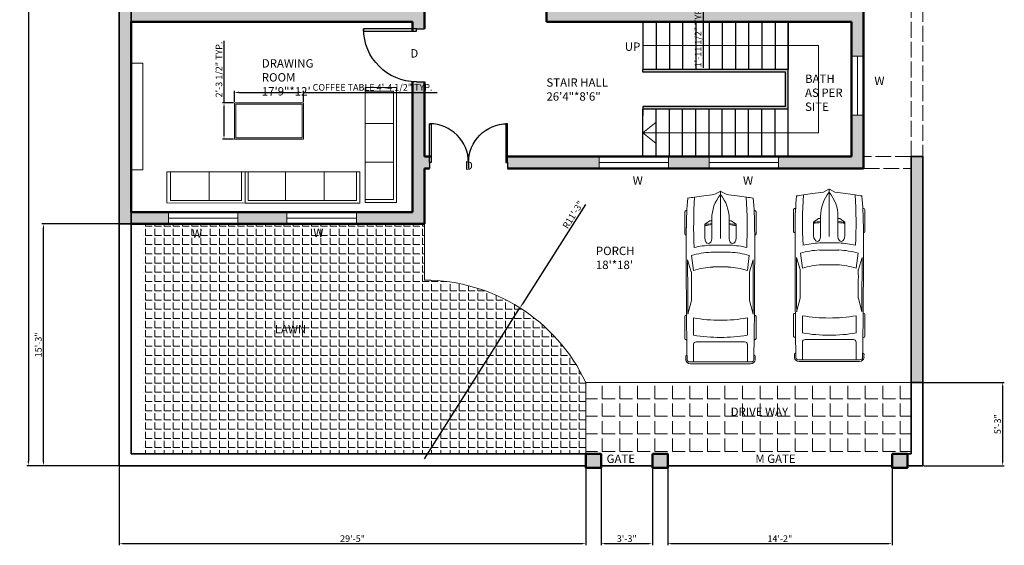
# Model space of a CAD drawing. Units: inches. Extents: x 554 to 1300, y 1707 to 2873.
# Tile 1 of 3: x 554 to 1300, y 1707 to 2105. Entities that reach past the tile are written whole.
import ezdxf

# ---------------------------------------------------------------- set-up
doc = ezdxf.new("R2010")
doc.units = ezdxf.units.IN
doc.linetypes.add('ACAD_ISO02W100', pattern=[15, 12, -3])
for name, color, linetype, lineweight in [('A-ANNO-DIMS', 145, 'Continuous', 18), ('A-ANNO-PATT', 7, 'Continuous', 13), ('A-ANNO-SYMB', 7, 'Continuous', 18), ('A-AREA-IDEN', 145, 'Continuous', 25), ('A-FLOR-STRS', 8, 'Continuous', 25), ('A-WALL-OVHD', 30, 'ACAD_ISO02W100', 18), ('A-WALL-PATT', 30, 'Continuous', 13), ('C-PKG-VEHI', 8, 'Continuous', 18), ('C-PROP', 30, 'Continuous', 35), ('C-PROP-OVHD', 30, 'ACAD_ISO02W100', 18), ('C-PVMT', 8, 'Continuous', 18), ('C-PVMT-PATT', 116, 'Continuous', 13), ('COLUMN', 30, 'Continuous', 50), ('DOOR', 52, 'Continuous', 25), ('FUR', 210, 'Continuous', 18), ('L-PLNT', 3, 'Continuous', 18), ('L-PLNT-PATT', 116, 'Continuous', 13), ('TEXT', 145, 'Continuous', 18), ('WALL', 30, 'Continuous', 50), ('WIND', 70, 'Continuous', 18)]:
    doc.layers.add(name, color=color, linetype=linetype, lineweight=lineweight)
doc.styles.get("Standard").update_dxf_attribs({"font": 'arial.ttf'})
doc.dimstyles.new('ISO-25', dxfattribs={"dimtxt": 5, "dimasz": 3.5, "dimexe": 1.25, "dimexo": 0.625, "dimtad": 1, "dimdec": 0, "dimlunit": 4, "dimtxsty": 'Standard', "dimcen": 2.5, "dimadec": 0, "dimazin": 0, "dimtfac": 1, "dimtdec": 0, "dimtmove": 0, "dimatfit": 3, "dimfxl": 1, "dimarcsym": 0})

# ---------------------------------------------------------------- blocks, each defined once
blk = doc.blocks.new('*U2')
for p, q in [((0, 0), (0, -6)), ((40, 0), (40, -6))]:
    blk.add_line(p, q)
blk.add_lwpolyline([(0, 0), (0, 40), (1.75, 40), (1.75, 0)], close=True)
blk.add_arc((0, 0), 40, 0, 90)
blk = doc.blocks.new('*U6')
for p, q in [((21.1, 37.4), (21.1, 36.8)), ((46.6, 38.9), (22.4, 38.9)), ((47.8, 37.4), (47.8, 37.4)), ((88, 31.9), (74.8, 35.9)), ((134.3, 35.6), (119.3, 31.8)), ((135.5, 37.1), (135.5, 37.4)), ((136.7, 38.9), (160.9, 38.9)), ((162.1, 37.4), (162.1, 36.8)), ((186.5, -33.5), (186.5, 33.5)), ((188.4, -32.8), (188.4, 32.8)), ((70, 31.5), (86.4, 29.4)), ((138.4, 29.4), (157.2, 29.4)), ((164.5, 26.4), (164.5, -26.4)), ((186.5, 29.4), (167, 29.4)), ((32.1, 9.5), (32.1, 11.2)), ((32.3, 11.6), (36.1, 17.2)), ((36.1, 17.2), (50.9, 17.2)), ((58.9, -10.8), (58.9, 10.8)), ((3.3, 6.1), (0.1, 0.4)), ((29.8, 9.5), (51.7, 9.5)), ((66.6, -10.5), (66.6, 10.5)), ((82.7, 8.5), (82.7, -8.5)), ((186.5, -10.5), (186.5, 10.5)), ((0, 0), (51.7, 0)), ((0.1, -0.4), (3.3, -6.1)), ((29.8, -9.5), (51.7, -9.5)), ((32.1, -9.5), (32.1, -11.2)), ((32.3, -11.6), (36.1, -17.2)), ((36.1, -17.2), (50.9, -17.2)), ((86.4, -29.4), (70, -31.5)), ((88, -31.9), (74.8, -35.9)), ((134.3, -35.6), (119.3, -31.8)), ((157.2, -29.4), (138.4, -29.4)), ((167, -29.4), (186.5, -29.4)), ((21.1, -37.4), (21.1, -36.8)), ((46.6, -38.9), (22.4, -38.9)), ((47.8, -37.4), (47.8, -37.4)), ((135.5, -37.1), (135.5, -37.4)), ((136.7, -38.9), (160.9, -38.9)), ((162.1, -37.4), (162.1, -36.8))]:
    blk.add_line(p, q)
for centre, major_axis, ratio, start_param, end_param in [((266, -27.5), (0, 313.3), 0.842304, 1.367076, 1.39176), ((41.2, -490.9), (0, 528.2), 0.842304, 0.00281, 0.075598), ((22.4, 37.4), (0, -1.48), 0.842304, 3.141593, 4.712389), ((64.5, -10555.6), (0, 10593), 0.842304, -0.013397, 0.002797), ((46.6, 37.4), (0, 1.48), 0.842304, -1.570796, 0), ((64.5, -10555.6), (0, -10591.5), 0.842304, 3.133765, 3.140441), ((136.7, 37.4), (0, -1.48), 0.842304, 3.141593, 4.712389), ((160.9, 37.4), (0, 1.48), 0.842304, -1.570796, 0), ((180.6, 35.8), (0, 2.22), 0.842304, -0.013017, 1.249894), ((64.5, -10556.4), (0, 10595.3), 0.842304, -0.013397, -0.013017), ((184, 32.8), (0, -5.25), 0.842304, 1.570796, 3.128196), ((184, 33.5), (0, -2.96), 0.842304, 1.570796, 3.128196), ((259.2, -27.5), (0, -305.3), 0.842304, 4.528606, 4.561838), ((37.5, -594), (0, -623.3), 0.842304, 3.096046, 3.200911), ((134.4, 5.4), (0, -89.8), 0.842304, 4.449482, 4.652344), ((135.3, 5.4), (0, 81.8), 0.842304, 1.245306, 1.50788), ((149.6, 2.8), (0, -79.6), 0.842304, 4.372215, 4.640744), ((95.8, -3666.4), (0, -3698.2), 0.842304, 3.134049, 3.144098), ((17.1, 0), (0, 147), 0.842304, 4.511394, 4.913384), ((35.9, 0), (0, 147), 0.842304, 4.511394, 4.913384), ((167, 26.4), (0, 2.96), 0.842304, 0, 1.570796), ((-204.5, 52.4), (0, -251), 0.842304, 1.385369, 1.434372), ((32.7, 11.2), (0, 0.74), 0.842304, 0.879714, 1.570796), ((13, 17), (0, 27.4), 0.842304, 4.435146, 4.718221), ((14.2, 17), (0, 27.4), 0.842304, 4.435146, 4.718221), ((50.8, 13.3), (6.34, -0.36), 0.603834, -1.395552, 1.581315), ((0.6, 0), (0, -0.74), 0.842304, 4.131459, 5.293319), ((29.8, -46.7), (0, 56.2), 0.842304, 0, 0.590319), ((-204.5, -52.4), (0, 251), 0.842304, -1.434372, -1.385369), ((29.8, 46.7), (0, 56.2), 0.842304, 2.551274, 3.141593), ((13, -17), (0, -27.4), 0.842304, 1.564964, 1.848039), ((14.2, -17), (0, -27.4), 0.842304, 1.564964, 1.848039), ((135.3, -5.4), (0, -81.8), 0.842304, -1.50788, -1.245306), ((149.6, -2.8), (0, -79.6), 0.842304, -1.499151, -1.230623), ((259.2, 27.5), (0, 305.3), 0.842304, 1.721348, 1.754579), ((32.7, -11.2), (0, -0.74), 0.842304, 4.712389, 5.403472), ((134.4, -5.4), (0, -89.8), 0.842304, -1.510751, -1.307889), ((266, 27.5), (0, 313.3), 0.842304, 1.749832, 1.774517), ((37.5, 594), (0, -623.3), 0.842304, -0.059319, 0.045547), ((95.8, 3666.4), (0, -3698.2), 0.842304, -0.002505, 0.007544), ((167, -26.4), (0, -2.96), 0.842304, 4.712389, 6.283185), ((41.2, 490.9), (0, -528.2), 0.842304, -0.075598, -0.00281), ((22.4, -37.4), (0, 1.48), 0.842304, 1.570796, 3.141593), ((64.5, 10555.6), (0, 10593), 0.842304, 3.138796, 3.15499), ((46.6, -37.4), (0, -1.48), 0.842304, 0, 1.570796), ((64.5, 10555.6), (0, -10591.5), 0.842304, 0.001152, 0.007828), ((136.7, -37.4), (0, -1.48), 0.842304, -1.570796, 0), ((160.9, -37.4), (0, 1.48), 0.842304, 3.141593, 4.712389), ((180.6, -35.8), (0, -2.22), 0.842304, -1.249894, 0.013017), ((64.5, 10556.4), (0, 10595.3), 0.842304, 3.15461, 3.15499), ((184, -32.8), (0, -5.25), 0.842304, 0.013397, 1.570796), ((184, -33.5), (0, 2.96), 0.842304, 3.15499, 4.712389)]:
    blk.add_ellipse(centre, major_axis=major_axis, ratio=ratio, start_param=start_param, end_param=end_param)
at = {"extrusion": (0, 0, -1)}
blk.add_ellipse((50.8, -13.3), major_axis=(6.34, 0.36), ratio=0.603834, start_param=-1.395552, end_param=1.581315, dxfattribs=at)
blk = doc.blocks.new('*D8')
at = {"layer": 'A-ANNO-DIMS', "color": 0, "lineweight": -2, "transparency": 16777216}
for p, q in [((629.06, 2841.48), (559.64, 2841.48)), ((560.89, 2837.98), (560.89, 1770.98)), ((629.06, 1767.48), (559.64, 1767.48))]:
    blk.add_line(p, q, dxfattribs=at)
at = {"layer": 'A-ANNO-DIMS', "color": 0, "lineweight": 100, "transparency": 16777216}
for points in [[(560.3, 2837.98), (561.47, 2837.98), (560.89, 2841.48)], [(560.3, 1770.98), (561.47, 1770.98), (560.89, 1767.48)]]:
    blk.add_solid(points, dxfattribs=at)
at = {"layer": 'Defpoints', "color": 0, "lineweight": 100, "transparency": 16777216}
for p in [(629.68, 2841.48), (560.89, 1767.48), (629.68, 1767.48)]:
    blk.add_point(p, dxfattribs=at)
at = {"layer": 'A-ANNO-DIMS', "color": 0, "transparency": 16777216, "insert": (557.71, 2304.48), "char_height": 5, "attachment_point": 5, "rotation": 90}
blk.add_mtext('89\'-6"', dxfattribs=at)
blk = doc.blocks.new('SOFA-3SEAT')
for p, q in [((0, 84.31), (0, 87)), ((0, 87), (23.69, 87)), ((23.69, 87), (23.69, 0)), ((0, 59.83), (21.61, 59.83)), ((0, 30.66), (21.61, 30.66)), ((0, 0), (0, 5.47)), ((23.69, 0), (0, 0))]:
    blk.add_line(p, q)
blk.add_lwpolyline([(21.61, 84.31), (0, 84.31), (0, 2.38), (21.61, 2.38)], close=True)
blk = doc.blocks.new('TABLE-COFFEE')
for points in [[(52.29, 0), (0, 0), (0, 27.46), (52.29, 27.46)], [(51.29, 1), (1, 1), (1, 26.46), (51.29, 26.46)]]:
    blk.add_lwpolyline(points, close=True)
blk = doc.blocks.new('*D17')
at = {"layer": 'A-ANNO-DIMS', "color": 0, "lineweight": -2, "transparency": 16777216}
for p, q in [((1059.32, 2142.65), (1073, 2142.65)), ((1071.75, 2139.15), (1071.75, 2122.46)), ((1059.32, 2118.96), (1073, 2118.96)), ((1071.75, 2118.96), (1071.75, 2068.67))]:
    blk.add_line(p, q, dxfattribs=at)
at = {"layer": 'A-ANNO-DIMS', "color": 0, "lineweight": 100, "transparency": 16777216}
for points in [[(1071.16, 2139.15), (1072.33, 2139.15), (1071.75, 2142.65)], [(1071.16, 2122.46), (1072.33, 2122.46), (1071.75, 2118.96)]]:
    blk.add_solid(points, dxfattribs=at)
at = {"layer": 'Defpoints', "color": 0, "lineweight": 100, "transparency": 16777216}
for p in [(1058.7, 2142.65), (1058.7, 2118.96), (1071.75, 2118.96)]:
    blk.add_point(p, dxfattribs=at)
at = {"layer": 'A-ANNO-DIMS', "color": 0, "transparency": 16777216, "insert": (1068.54, 2092.06), "char_height": 5, "attachment_point": 5, "rotation": 90}
blk.add_mtext('1\'-11 1/2" TYP.', dxfattribs=at)
blk = doc.blocks.new('*D26')
at = {"layer": 'A-ANNO-DIMS', "color": 0, "lineweight": -2, "transparency": 16777216}
for p, q in [((716.83, 2042.82), (716.83, 2051.29)), ((720.33, 2050.04), (765.63, 2050.04)), ((769.13, 2042.82), (769.13, 2051.29)), ((769.13, 2050.04), (870.29, 2050.04))]:
    blk.add_line(p, q, dxfattribs=at)
at = {"layer": 'A-ANNO-DIMS', "color": 0, "lineweight": 100, "transparency": 16777216}
for points in [[(720.33, 2050.62), (720.33, 2049.46), (716.83, 2050.04)], [(765.63, 2050.62), (765.63, 2049.46), (769.13, 2050.04)]]:
    blk.add_solid(points, dxfattribs=at)
at = {"layer": 'Defpoints', "color": 0, "lineweight": 100, "transparency": 16777216}
for p in [(769.13, 2050.04), (716.83, 2042.2), (769.13, 2042.2)]:
    blk.add_point(p, dxfattribs=at)
at = {"layer": 'A-ANNO-DIMS', "color": 0, "transparency": 16777216, "insert": (821.46, 2053.25), "char_height": 5, "attachment_point": 5}
blk.add_mtext('COFFEE TABLE 4\'-4 1/2" TYP.', dxfattribs=at)
blk = doc.blocks.new('*D27')
at = {"layer": 'A-ANNO-DIMS', "color": 0, "lineweight": -2, "transparency": 16777216}
for p, q in [((708.99, 2042.2), (708.99, 2089.16)), ((716.21, 2042.2), (707.74, 2042.2)), ((708.99, 2018.24), (708.99, 2038.7)), ((716.21, 2014.74), (707.74, 2014.74))]:
    blk.add_line(p, q, dxfattribs=at)
at = {"layer": 'A-ANNO-DIMS', "color": 0, "lineweight": 100, "transparency": 16777216}
for points in [[(708.41, 2038.7), (709.57, 2038.7), (708.99, 2042.2)], [(708.41, 2018.24), (709.57, 2018.24), (708.99, 2014.74)]]:
    blk.add_solid(points, dxfattribs=at)
at = {"layer": 'Defpoints', "color": 0, "lineweight": 100, "transparency": 16777216}
for p in [(708.99, 2042.2), (716.83, 2042.2), (716.83, 2014.74)]:
    blk.add_point(p, dxfattribs=at)
at = {"layer": 'A-ANNO-DIMS', "color": 0, "transparency": 16777216, "insert": (705.78, 2067.43), "char_height": 5, "attachment_point": 5, "rotation": 90}
blk.add_mtext('2\'-3 1/2" TYP.', dxfattribs=at)
blk = doc.blocks.new('*D30')
at = {"layer": 'A-ANNO-DIMS', "color": 0, "lineweight": -2, "transparency": 16777216}
for p, q in [((629.06, 1950.48), (571.03, 1950.48)), ((572.28, 1770.98), (572.28, 1946.98)), ((629.06, 1767.48), (571.03, 1767.48))]:
    blk.add_line(p, q, dxfattribs=at)
at = {"layer": 'A-ANNO-DIMS', "color": 0, "lineweight": 100, "transparency": 16777216}
for points in [[(571.7, 1946.98), (572.86, 1946.98), (572.28, 1950.48)], [(571.7, 1770.98), (572.86, 1770.98), (572.28, 1767.48)]]:
    blk.add_solid(points, dxfattribs=at)
at = {"layer": 'Defpoints', "color": 0, "lineweight": 100, "transparency": 16777216}
for p in [(572.28, 1950.48), (629.68, 1950.48), (629.68, 1767.48)]:
    blk.add_point(p, dxfattribs=at)
at = {"layer": 'A-ANNO-DIMS', "color": 0, "transparency": 16777216, "insert": (569.1, 1858.98), "char_height": 5, "attachment_point": 5, "rotation": 90}
blk.add_mtext('15\'-3"', dxfattribs=at)
blk = doc.blocks.new('*D31')
at = {"layer": 'A-ANNO-DIMS', "color": 0, "lineweight": -2, "transparency": 16777216}
for p, q in [((629.68, 1766.85), (629.68, 1707.27)), ((982.92, 1766.85), (982.92, 1707.27)), ((633.18, 1708.52), (979.42, 1708.52))]:
    blk.add_line(p, q, dxfattribs=at)
at = {"layer": 'A-ANNO-DIMS', "color": 0, "lineweight": 100, "transparency": 16777216}
for points in [[(633.18, 1709.1), (633.18, 1707.94), (629.68, 1708.52)], [(979.42, 1709.1), (979.42, 1707.94), (982.92, 1708.52)]]:
    blk.add_solid(points, dxfattribs=at)
at = {"layer": 'Defpoints', "color": 0, "lineweight": 100, "transparency": 16777216}
for p in [(629.68, 1767.48), (982.92, 1767.48), (982.92, 1708.52)]:
    blk.add_point(p, dxfattribs=at)
at = {"layer": 'A-ANNO-DIMS', "color": 0, "transparency": 16777216, "insert": (806.3, 1711.7), "char_height": 5, "attachment_point": 5}
blk.add_mtext('29\'-5"', dxfattribs=at)
blk = doc.blocks.new('*D32')
at = {"layer": 'A-ANNO-DIMS', "color": 0, "lineweight": -2, "transparency": 16777216}
for p, q in [((994.52, 1766.85), (994.52, 1707.27)), ((1033.28, 1766.85), (1033.28, 1707.27)), ((998.02, 1708.52), (1029.78, 1708.52))]:
    blk.add_line(p, q, dxfattribs=at)
at = {"layer": 'A-ANNO-DIMS', "color": 0, "lineweight": 100, "transparency": 16777216}
for points in [[(998.02, 1709.1), (998.02, 1707.94), (994.52, 1708.52)], [(1029.78, 1709.1), (1029.78, 1707.94), (1033.28, 1708.52)]]:
    blk.add_solid(points, dxfattribs=at)
at = {"layer": 'Defpoints', "color": 0, "lineweight": 100, "transparency": 16777216}
for p in [(994.52, 1767.48), (1033.28, 1767.48), (1033.28, 1708.52)]:
    blk.add_point(p, dxfattribs=at)
at = {"layer": 'A-ANNO-DIMS', "color": 0, "transparency": 16777216, "insert": (1013.9, 1711.7), "char_height": 5, "attachment_point": 5}
blk.add_mtext('3\'-3"', dxfattribs=at)
blk = doc.blocks.new('*D33')
at = {"layer": 'A-ANNO-DIMS', "color": 0, "lineweight": -2, "transparency": 16777216}
for p, q in [((1044.88, 1766.85), (1044.88, 1707.27)), ((1214.77, 1766.85), (1214.77, 1707.27)), ((1048.38, 1708.52), (1211.27, 1708.52))]:
    blk.add_line(p, q, dxfattribs=at)
at = {"layer": 'A-ANNO-DIMS', "color": 0, "lineweight": 100, "transparency": 16777216}
for points in [[(1048.38, 1709.1), (1048.38, 1707.94), (1044.88, 1708.52)], [(1211.27, 1709.1), (1211.27, 1707.94), (1214.77, 1708.52)]]:
    blk.add_solid(points, dxfattribs=at)
at = {"layer": 'Defpoints', "color": 0, "lineweight": 100, "transparency": 16777216}
for p in [(1044.88, 1767.48), (1214.77, 1767.48), (1214.77, 1708.52)]:
    blk.add_point(p, dxfattribs=at)
at = {"layer": 'A-ANNO-DIMS', "color": 0, "transparency": 16777216, "insert": (1129.82, 1711.66), "char_height": 5, "attachment_point": 5}
blk.add_mtext('14\'-2"', dxfattribs=at)
blk = doc.blocks.new('*D34')
at = {"layer": 'A-ANNO-DIMS', "color": 0, "lineweight": -2, "transparency": 16777216}
for p, q in [((1238.81, 1830.48), (1299.75, 1830.48)), ((1298.5, 1826.98), (1298.5, 1770.98)), ((1238.81, 1767.48), (1299.75, 1767.48))]:
    blk.add_line(p, q, dxfattribs=at)
at = {"layer": 'A-ANNO-DIMS', "color": 0, "lineweight": 100, "transparency": 16777216}
for points in [[(1297.91, 1826.98), (1299.08, 1826.98), (1298.5, 1830.48)], [(1297.91, 1770.98), (1299.08, 1770.98), (1298.5, 1767.48)]]:
    blk.add_solid(points, dxfattribs=at)
at = {"layer": 'Defpoints', "color": 0, "lineweight": 100, "transparency": 16777216}
for p in [(1238.18, 1830.48), (1238.18, 1767.48), (1298.5, 1767.48)]:
    blk.add_point(p, dxfattribs=at)
at = {"layer": 'A-ANNO-DIMS', "color": 0, "transparency": 16777216, "insert": (1295.32, 1798.98), "char_height": 5, "attachment_point": 5, "rotation": 90}
blk.add_mtext('5\'-3"', dxfattribs=at)
blk = doc.blocks.new('*D36')
at = {"layer": 'A-ANNO-DIMS', "color": 0, "lineweight": -2, "transparency": 16777216}
for p, q in [((982.68, 1965.25), (934.92, 1889.93)), ((860.68, 1772.83), (933.05, 1886.97))]:
    blk.add_line(p, q, dxfattribs=at)
at = {"layer": 'A-ANNO-DIMS', "color": 0, "lineweight": 100, "transparency": 16777216}
blk.add_solid([(934.43, 1890.24), (935.41, 1889.61), (933.05, 1886.97)], dxfattribs=at)
at = {"layer": 'Defpoints', "color": 0, "lineweight": 100, "transparency": 16777216}
for p in [(933.05, 1886.97), (860.68, 1772.83)]:
    blk.add_point(p, dxfattribs=at)
at = {"layer": 'A-ANNO-DIMS', "color": 0, "transparency": 16777216, "insert": (973.78, 1957.16), "char_height": 5, "attachment_point": 5, "rotation": 57.62466}
blk.add_mtext('R11\'-3"', dxfattribs=at)

msp = doc.modelspace()

# ---------------------------------------------------------------- hatches: boundary and pattern name
at = {"layer": 'A-ANNO-PATT'}
h = msp.add_hatch(dxfattribs=at)
h.set_pattern_fill('ACAD_ISO04W100', color=256, scale=1.9)
h.paths.add_polyline_path([(1036.18, 2027.51), (1026.18, 2019.48), (1036.18, 2019.48)])
h.paths.add_polyline_path([(1036.18, 2019.48), (1026.18, 2019.48), (1036.18, 2011.45)])
h = msp.add_hatch(dxfattribs=at)
h.set_pattern_fill('ACAD_ISO04W100', color=256, scale=1.9)
h.paths.add_polyline_path([(1036.18, 2027.51), (1026.18, 2019.48), (1036.18, 2019.48)])
h.paths.add_polyline_path([(1036.18, 2019.48), (1026.18, 2019.48), (1036.18, 2011.45)])
at = {"layer": 'A-WALL-PATT'}
h = msp.add_hatch(color=256, dxfattribs=at)
h.dxf.hatch_style = 1
h.paths.add_polyline_path([(1136.18, 2067.48), (1026.18, 2067.48), (1026.18, 2065.48), (1134.18, 2065.48), (1134.18, 2039.48), (1026.18, 2039.48), (1026.18, 2037.48), (1136.18, 2037.48)])
h.paths.add_polyline_path([(1193.18, 2103.48), (1184.18, 2103.48), (1184.18, 2077.52), (1193.18, 2077.52)])
h.paths.add_polyline_path([(1193.18, 2032.94), (1184.18, 2032.94), (1184.18, 2001.48), (1148.18, 2001.48), (1136.18, 2001.48), (1128.74, 2001.48), (1128.74, 1992.48), (1193.18, 1992.48), (1193.18, 2001.48)])
h.paths.add_polyline_path([(1076.18, 2001.48), (1045.59, 2001.48), (1045.59, 1992.48), (1076.18, 1992.48)])
h.paths.add_polyline_path([(993.02, 2001.48), (923.53, 2001.48), (923.53, 1996.9), (923.53, 1992.48), (993.02, 1992.48)])
h.paths.add_polyline_path([(1184.18, 2112.48), (962.18, 2112.48), (962.18, 2151.15), (953.18, 2151.15), (953.18, 2103.48), (1184.18, 2103.48)])
h.paths.add_polyline_path([(1193.18, 2144.33), (1184.18, 2144.33), (1184.18, 2112.48), (1184.18, 2103.48), (1193.18, 2103.48)])
h.paths.add_polyline_path([(772.18, 2796.48), (758.22, 2796.48), (758.22, 2787.48), (767.68, 2787.48), (772.18, 2787.48)])
h.paths.add_polyline_path([(737.06, 2796.48), (674.68, 2796.48), (674.68, 2710.98), (683.68, 2710.98), (683.68, 2715.48), (683.68, 2787.48), (737.06, 2787.48)])
h.paths.add_polyline_path([(786.15, 2796.48), (772.18, 2796.48), (772.18, 2787.48), (786.15, 2787.48)])
h.paths.add_polyline_path([(860.68, 2796.48), (807.31, 2796.48), (807.31, 2787.48), (856.18, 2787.48), (860.68, 2787.48)])
h.paths.add_polyline_path([(905.53, 2796.48), (860.68, 2796.48), (860.68, 2787.48), (905.53, 2787.48)])
h.paths.add_polyline_path([(860.68, 2787.48), (856.18, 2787.48), (856.18, 2715.48), (853.67, 2715.48), (853.67, 2713.96), (853.67, 2710.98), (856.18, 2710.98), (860.68, 2710.98)])
h.paths.add_polyline_path([(772.18, 2787.48), (767.68, 2787.48), (767.68, 2715.48), (728.12, 2715.48), (706.98, 2715.48, -0.019152), (707.04, 2713.96), (707.04, 2710.98), (772.18, 2710.98)])
h.paths.add_polyline_path([(833.86, 2715.48), (772.18, 2715.48), (772.18, 2710.98), (833.8, 2710.98), (833.8, 2713.96, -0.019152)])
h.paths.add_polyline_path([(1025.68, 2796.48), (981.39, 2796.48), (981.39, 2787.48), (1001.03, 2787.48), (1016.68, 2787.48), (1025.68, 2787.48)])
h.paths.add_polyline_path([(1094.68, 2796.48), (1025.68, 2796.48), (1025.68, 2787.48), (1085.68, 2787.48), (1094.68, 2787.48)])
h.paths.add_polyline_path([(1140.18, 2796.48), (1094.68, 2796.48), (1094.68, 2787.48), (1140.18, 2787.48)], flags=17)
h.paths.add_polyline_path([(1185.68, 2796.48), (1161.35, 2796.48), (1161.35, 2787.48), (1176.68, 2787.48), (1176.68, 2736.68), (1176.72, 2736.68), (1176.72, 2715.48), (1137.16, 2715.48), (1094.68, 2715.48), (1094.68, 2706.48), (1185.68, 2706.48)])
h.paths.add_polyline_path([(1094.68, 2787.48), (1085.68, 2787.48), (1085.68, 2748.92), (1090.01, 2748.92, -0.040642), (1094.68, 2748.54)])
h.paths.add_polyline_path([(1025.68, 2787.48), (1016.68, 2787.48), (1016.68, 2607.48), (1016.68, 2598.48), (1025.68, 2598.48), (1025.68, 2672.36), (1025.68, 2706.48)])
h.paths.add_polyline_path([(1094.68, 2715.48), (1094.68, 2720.05), (1090.01, 2720.05), (1085.68, 2720.05), (1085.68, 2715.48), (1082.66, 2715.48), (1082.66, 2706.48), (1094.68, 2706.48)])
h.paths.add_polyline_path([(1043.78, 2715.48), (1025.68, 2715.48), (1025.68, 2706.48), (1043.78, 2706.48)])
h.paths.add_polyline_path([(1185.68, 2577.7), (1176.68, 2577.7), (1176.68, 2570), (1176.68, 2526.48), (1176.68, 2517.48), (1185.68, 2517.48)])
h.paths.add_polyline_path([(1185.68, 2706.48), (1176.68, 2706.48), (1176.68, 2670.52), (1185.68, 2670.52)])
h.paths.add_polyline_path([(1025.68, 2598.48), (1016.68, 2598.48), (1016.68, 2569.99), (1022.68, 2569.99, -0.01877), (1025.68, 2569.88)])
h.paths.add_polyline_path([(1016.68, 2607.48), (903.83, 2607.48, -0.01877), (903.94, 2604.48), (903.94, 2598.48), (1016.68, 2598.48)])
h.paths.add_polyline_path([(860.68, 2646.48), (851.68, 2646.48), (851.68, 2508.85, -0.01877), (854.68, 2508.96), (860.68, 2508.96)])
h.paths.add_polyline_path([(863.94, 2604.48), (863.94, 2607.48), (860.68, 2607.48), (860.68, 2598.48), (863.94, 2598.48)])
h.paths.add_polyline_path([(1101.44, 2750.41), (1134.65, 2750.41), (1134.65, 2774.1), (1101.44, 2774.1)], flags=25)
h.paths.add_polyline_path([(1049.21, 2750.31), (1082.94, 2750.31), (1082.94, 2773.99), (1049.21, 2773.99)], flags=9)
h = msp.add_hatch(color=256, dxfattribs=at)
h.dxf.hatch_style = 1
h.paths.add_polyline_path([(683.68, 2710.98), (674.68, 2710.98), (674.68, 2646.48), (674.68, 2589.67), (683.68, 2589.67), (683.68, 2646.48), (683.68, 2650.98)])
h.paths.add_polyline_path([(688.17, 2650.98), (683.68, 2650.98), (683.68, 2646.48), (688.17, 2646.48)])
h.paths.add_polyline_path([(772.18, 2710.98), (767.68, 2710.98), (767.68, 2650.98), (730.85, 2650.98), (730.85, 2646.48), (772.18, 2646.48)])
h.paths.add_polyline_path([(860.68, 2710.98), (856.18, 2710.98), (856.18, 2650.98), (772.18, 2650.98), (772.18, 2646.48), (860.68, 2646.48)])
h.paths.add_polyline_path([(683.68, 2496.84), (674.68, 2496.84), (674.68, 2445.48), (683.68, 2445.48), (683.68, 2454.48)])
h.paths.add_polyline_path([(851.68, 2454.48), (683.68, 2454.48), (683.68, 2445.48), (851.68, 2445.48)])
h.paths.add_polyline_path([(707.68, 2445.48), (698.68, 2445.48), (698.68, 2419.1), (707.68, 2419.1)])
h.paths.add_polyline_path([(698.68, 2289.48), (687.57, 2289.48), (687.57, 2280.48), (696.57, 2280.48), (698.68, 2280.48)])
h.paths.add_polyline_path([(687.57, 2217.48), (671.17, 2217.48), (671.17, 2208.48), (687.57, 2208.48)])
h.paths.add_polyline_path([(650.01, 2217.48), (638.68, 2217.48), (638.68, 2208.48), (650.01, 2208.48)])
h.paths.add_polyline_path([(860.68, 2235.34), (854.68, 2235.34, -0.01877), (851.68, 2235.45), (851.68, 2112.48), (696.57, 2112.48), (696.57, 2103.48), (860.68, 2103.48)])
h.paths.add_polyline_path([(666.88, 1959.48), (647.68, 1959.48), (638.68, 1959.48), (638.68, 1950.48), (647.68, 1950.48), (666.88, 1950.48)])
h.paths.add_polyline_path([(756.66, 1959.48), (719.44, 1959.48), (719.44, 1950.48), (756.66, 1950.48)])
h.paths.add_polyline_path([(860.68, 1992.48), (864.62, 1992.48), (864.62, 1996.9), (864.62, 2001.48), (860.68, 2001.48), (860.68, 2058.13), (854.68, 2058.13, -0.01877), (851.68, 2058.24), (851.68, 1992.48), (851.68, 1959.48), (809.22, 1959.48), (809.22, 1950.48), (860.68, 1950.48)])
h.paths.add_polyline_path([(860.68, 2103.48), (851.68, 2103.48), (851.68, 2098.13), (854.68, 2098.13), (860.68, 2098.13)])
h.paths.add_polyline_path([(984.68, 2397.2), (984.68, 2469.19, -0.01877), (981.68, 2469.08), (975.68, 2469.08), (975.68, 2361.48), (975.68, 2355.65), (984.68, 2355.65), (984.68, 2361.48), (984.68, 2370.48)])
h.paths.add_polyline_path([(1109.18, 2409.48), (1104.68, 2409.48), (1104.68, 2370.48), (984.68, 2370.48), (984.68, 2361.48), (1109.18, 2361.48)])
h.paths.add_polyline_path([(1125.26, 2418.48), (1109.18, 2418.48), (1109.18, 2488.51), (1105.47, 2488.51, -0.008003), (1104.68, 2488.52), (1104.68, 2409.48), (1109.18, 2409.48), (1125.26, 2409.48)])
h.paths.add_polyline_path([(1185.68, 2418.48), (1167, 2418.48), (1167, 2409.48), (1185.68, 2409.48)])
h.paths.add_polyline_path([(1185.68, 2488.51), (1181.97, 2488.51, -0.008003), (1181.18, 2488.52), (1181.18, 2418.48), (1185.68, 2418.48)])
h.paths.add_polyline_path([(1025.68, 2529.99), (1022.68, 2529.99), (1016.68, 2529.99), (1016.68, 2526.48), (975.68, 2526.48), (975.68, 2517.48), (1025.68, 2517.48)])
h.paths.add_polyline_path([(984.68, 2517.48), (975.68, 2517.48), (975.68, 2509.08), (981.68, 2509.08), (984.68, 2509.08)])
h.paths.add_polyline_path([(1176.68, 2526.48), (1025.68, 2526.48), (1025.68, 2517.48), (1104.68, 2517.48), (1176.68, 2517.48)])
h.paths.add_polyline_path([(745.17, 1864.25), (773.96, 1864.25), (773.96, 1877.33), (745.17, 1877.33)], flags=9)
h = msp.add_hatch(color=256, dxfattribs=at)
h.dxf.hatch_style = 1
h.paths.add_polyline_path([(638.68, 2072.33), (638.68, 2103.48), (638.68, 2217.48), (629.68, 2217.48), (629.68, 2097.48), (629.68, 1992.48), (629.68, 1950.48), (638.68, 1950.48), (638.68, 1992.48)])
h.paths.add_polyline_path([(696.57, 2217.48), (687.57, 2217.48), (687.57, 2142.07, -0.048021), (692.61, 2142.55), (696.57, 2142.55)])
h.paths.add_polyline_path([(696.57, 2116.14), (692.61, 2116.14), (687.57, 2116.14), (687.57, 2112.48), (638.68, 2112.48), (638.68, 2103.48), (687.57, 2103.48), (696.57, 2103.48), (696.57, 2112.48)])
h.paths.add_polyline_path([(1010.14, 2078.06), (1025.63, 2078.06), (1025.63, 2091.14), (1010.14, 2091.14)], flags=9)
h.paths.add_polyline_path([(1129.91, 2440.07), (1172.04, 2440.07), (1172.04, 2474.45), (1129.91, 2474.45)], flags=9)
h.paths.add_polyline_path([(1022.04, 2432.2), (1064.45, 2432.2), (1064.45, 2455.89), (1022.04, 2455.89)], flags=9)
h.paths.add_polyline_path([(891.25, 2147.87), (936.31, 2147.87), (936.31, 2182.23), (891.25, 2182.23)], flags=9)
h.paths.add_polyline_path([(951.1, 2040.21), (1005.03, 2040.21), (1005.03, 2063.9), (951.1, 2063.9)], flags=9)
h.paths.add_polyline_path([(988, 1912.76), (1023.48, 1912.76), (1023.48, 1936.45), (988, 1936.45)], flags=9)
h.paths.add_polyline_path([(735.06, 2044.01), (781.37, 2044.01), (781.37, 2078.39), (735.06, 2078.39)], flags=9)
h.paths.add_polyline_path([(651.07, 2140.85), (677.89, 2140.85), (677.89, 2164.54), (651.07, 2164.54)], flags=9)
h.paths.add_polyline_path([(769.16, 2219.79), (818.47, 2219.79), (818.47, 2243.48), (769.16, 2243.48)], flags=9)
h.paths.add_polyline_path([(745.28, 2587.79), (794.59, 2587.79), (794.59, 2611.48), (745.28, 2611.48)], flags=9)
h = msp.add_hatch(color=256, dxfattribs=at)
h.dxf.hatch_style = 1
h.paths.add_polyline_path([(994.52, 1776.48), (982.92, 1776.48), (982.92, 1765.92), (994.52, 1765.92)])
h.paths.add_polyline_path([(1044.88, 1776.48), (1033.28, 1776.48), (1033.28, 1765.92), (1044.88, 1765.92)])
h.paths.add_polyline_path([(1226.37, 1776.48), (1214.77, 1776.48), (1214.77, 1765.92), (1226.37, 1765.92)])
h.paths.add_polyline_path([(1241.1, 2418.48), (1229.18, 2418.48), (1229.18, 2407.99), (1241.1, 2407.99)])
h.paths.add_polyline_path([(1241.1, 2290.97), (1229.18, 2290.97), (1229.18, 2280.48), (1238.18, 2280.48), (1241.1, 2280.48)])
h.paths.add_polyline_path([(1229.18, 2418.48), (1185.68, 2418.48), (1185.68, 2409.48), (1229.18, 2409.48)])
h.paths.add_polyline_path([(1229.18, 2289.48), (1089.68, 2289.48), (1089.68, 2280.48), (1110.8, 2280.48), (1184.18, 2280.48), (1193.18, 2280.48), (1229.18, 2280.48)])
h.paths.add_polyline_path([(1193.18, 2280.48), (1184.18, 2280.48), (1184.18, 2237.16), (1193.18, 2237.16)])
h.paths.add_polyline_path([(1089.68, 2289.48), (953.18, 2289.48), (953.18, 2280.48), (953.18, 2239.7), (962.18, 2239.7), (962.18, 2280.48), (1089.68, 2280.48)])
h.paths.add_polyline_path([(860.68, 2289.48), (851.68, 2289.48), (851.68, 2280.48), (860.68, 2280.48)])
h.paths.add_polyline_path([(860.68, 2280.48), (851.68, 2280.48), (851.68, 2275.34), (854.68, 2275.34), (860.68, 2275.34)])
h.paths.add_polyline_path([(860.68, 2445.48), (860.68, 2468.96), (854.68, 2468.96), (851.68, 2468.96), (851.68, 2454.48), (851.68, 2445.48), (851.68, 2289.48), (860.68, 2289.48)])
h.paths.add_polyline_path([(851.68, 2289.48), (707.68, 2289.48), (707.68, 2326.28), (698.68, 2326.28), (698.68, 2280.48), (851.68, 2280.48)])
h.paths.add_polyline_path([(1241.54, 2332.25), (1241.54, 2369.42), (1228.46, 2369.42), (1228.46, 2332.25)], flags=9)
h.paths.add_polyline_path([(1157.71, 2330.44), (1193.19, 2330.44), (1193.19, 2354.12), (1157.71, 2354.12)], flags=9)
h = msp.add_hatch(color=256, dxfattribs=at)
h.dxf.hatch_style = 1
h.paths.add_polyline_path([(1238.18, 1952.91), (1238.18, 2001.48), (1229.18, 2001.48), (1229.18, 1992.48), (1229.18, 1939.04), (1229.18, 1830.48), (1238.18, 1830.48)])
at = {"layer": 'C-PVMT-PATT'}
h = msp.add_hatch(dxfattribs=at)
h.set_pattern_fill('ANGLE', color=256, scale=1.9)
h.set_pattern_definition([(0, (0, 0), (0, 13.2715), [9.652, -3.6195]), (90, (0, 0), (-13.2715, 8e-16), [9.652, -3.6195])])
h.paths.add_polyline_path([(982.92, 1830.48), (982.92, 1776.48), (1229.18, 1776.48), (1229.18, 1830.48)])
at = {"layer": 'L-PLNT-PATT'}
h = msp.add_hatch(dxfattribs=at)
h.set_pattern_fill('ANGLE', color=256)
h.set_pattern_definition([(0, (0, 0), (0, 6.985), [5.08, -1.905]), (90, (0, 0), (-6.985, 4e-16), [5.08, -1.905])])
h.paths.add_polyline_path([(860.68, 1907.98), (860.68, 1950.48), (647.68, 1950.48), (647.68, 1848.48), (647.68, 1776.48), (982.92, 1776.48), (982.92, 1830.48, 0.290295)])

# ---------------------------------------------------------------- linework, layer by layer
at = {"layer": 'A-ANNO-SYMB'}
for p, q in [((1026.18, 2085.48), (1159.09, 2085.48)), ((1159.09, 2085.48), (1159.09, 2019.48)), ((1026.18, 2019.48), (1036.18, 2027.51)), ((1159.09, 2019.48), (1026.18, 2019.48)), ((1026.18, 2019.48), (1036.18, 2011.45))]:
    msp.add_line(p, q, dxfattribs=at)
at = {"layer": 'A-FLOR-STRS'}
for p, q in [((1026.18, 2103.48), (1026.18, 2067.48)), ((1036.18, 2103.48), (1036.18, 2067.48)), ((1046.18, 2103.48), (1046.18, 2067.48)), ((1056.18, 2103.48), (1056.18, 2067.48)), ((1066.18, 2103.48), (1066.18, 2067.48)), ((1076.18, 2103.48), (1076.18, 2067.48)), ((1086.18, 2103.48), (1086.18, 2067.48)), ((1096.18, 2103.48), (1096.18, 2067.48)), ((1106.18, 2103.48), (1106.18, 2067.48)), ((1116.18, 2103.48), (1116.18, 2067.48)), ((1126.18, 2103.48), (1126.18, 2067.48)), ((1136.18, 2001.48), (1136.18, 2103.48)), ((1136.18, 2103.48), (1136.18, 2067.48)), ((1136.18, 2067.48), (1026.18, 2067.48)), ((1026.18, 2065.48), (1026.18, 2067.48)), ((1134.18, 2065.48), (1026.18, 2065.48)), ((1134.18, 2039.48), (1134.18, 2065.48)), ((1134.18, 2039.48), (1026.18, 2039.48)), ((1026.18, 2039.48), (1026.18, 2032.57)), ((1136.18, 2037.48), (1026.18, 2037.48)), ((1026.18, 2001.48), (1026.18, 2037.48)), ((1036.18, 2001.48), (1036.18, 2037.48)), ((1046.18, 2001.48), (1046.18, 2037.48)), ((1056.18, 2001.48), (1056.18, 2037.48)), ((1066.18, 2001.48), (1066.18, 2037.48)), ((1076.18, 2001.48), (1076.18, 2037.48)), ((1086.18, 2001.48), (1086.18, 2037.48)), ((1096.18, 2001.48), (1096.18, 2037.48)), ((1106.18, 2001.48), (1106.18, 2037.48)), ((1116.18, 2001.48), (1116.18, 2037.48)), ((1126.18, 2001.48), (1126.18, 2037.48)), ((1136.18, 2001.48), (1136.18, 2037.48))]:
    msp.add_line(p, q, dxfattribs=at)
at = {"layer": 'A-WALL-OVHD'}
msp.add_lwpolyline([(1229.18, 2001.48), (1193.18, 2001.48), (1193.18, 1992.48), (1229.18, 1992.48)], close=True, dxfattribs=at)
at = {"layer": 'C-PROP'}
for p, q in [((629.68, 2841.48), (629.68, 2097.48)), ((638.68, 2832.48), (638.68, 2097.48)), ((629.68, 2097.48), (629.68, 1992.48)), ((638.68, 2097.48), (638.68, 2001.48)), ((638.68, 2001.48), (638.68, 1992.48)), ((1229.18, 2001.48), (1229.18, 1939.04)), ((1229.18, 2001.48), (1238.18, 2001.48)), ((1238.18, 2001.48), (1238.18, 1932.04)), ((629.68, 1992.48), (629.68, 1839.48)), ((638.68, 1992.48), (638.68, 1776.48)), ((638.68, 1950.48), (629.68, 1950.48)), ((1229.18, 1776.48), (1229.18, 1952.91)), ((1238.18, 1767.48), (1238.18, 1952.91)), ((629.68, 1767.48), (629.68, 1848.48)), ((1229.18, 1830.48), (1238.18, 1830.48)), ((638.68, 1776.48), (994.52, 1776.48)), ((1033.28, 1776.48), (1044.88, 1776.48)), ((1214.77, 1776.48), (1229.18, 1776.48)), ((982.92, 1767.48), (629.68, 1767.48)), ((1004.18, 1767.48), (994.52, 1767.48)), ((1004.18, 1767.48), (1033.28, 1767.48)), ((1044.88, 1767.48), (1214.77, 1767.48)), ((1226.37, 1767.48), (1238.18, 1767.48))]:
    msp.add_line(p, q, dxfattribs=at)
at = {"layer": 'C-PROP-OVHD'}
msp.add_lwpolyline([(1238.18, 2001.48), (1229.18, 2001.48), (1229.18, 2280.48), (1238.18, 2280.48)], close=True, dxfattribs=at)
at = {"layer": 'C-PVMT'}
msp.add_line((982.92, 1830.48), (1229.18, 1830.48), dxfattribs=at)
at = {"layer": 'COLUMN'}
for points in [[(982.92, 1776.48), (994.52, 1776.48), (994.52, 1765.92), (982.92, 1765.92)], [(1033.28, 1776.48), (1044.88, 1776.48), (1044.88, 1765.92), (1033.28, 1765.92)], [(1214.77, 1776.48), (1226.37, 1776.48), (1226.37, 1765.92), (1214.77, 1765.92)]]:
    msp.add_lwpolyline(points, close=True, dxfattribs=at)
at = {"layer": 'FUR'}
for p, q in [((668.58, 1989.96), (665.61, 1989.96)), ((665.61, 1989.96), (665.61, 1966.37)), ((668.58, 1989.96), (668.58, 1968.35)), ((697.75, 1989.96), (697.75, 1968.35)), ((722.22, 1989.96), (724.92, 1989.96)), ((724.92, 1989.96), (724.92, 1966.28)), ((724.92, 1966.28), (665.61, 1966.37))]:
    msp.add_line(p, q, dxfattribs=at)
msp.add_lwpolyline([(638.68, 2072.33), (638.68, 1991.47), (647.61, 1991.47), (647.61, 2072.33)], close=True, dxfattribs=at)
msp.add_lwpolyline([(668.58, 1968.35), (722.22, 1968.35), (722.22, 1989.96), (668.58, 1989.96)], dxfattribs=at)
at = {"layer": 'L-PLNT'}
for p, q in [((860.68, 1950.48), (860.68, 1907.98)), ((982.92, 1776.48), (982.92, 1830.48))]:
    msp.add_line(p, q, dxfattribs=at)
msp.add_arc((860.68, 1772.83), 135.15, 25.24908, 90, dxfattribs=at)
at = {"layer": 'WALL'}
for p, q in [((953.18, 2289.48), (953.18, 2103.48)), ((1193.18, 2280.48), (1193.18, 2103.48)), ((860.68, 2235.34), (860.68, 2103.48)), ((687.57, 2103.48), (638.68, 2103.48)), ((638.68, 2103.48), (638.68, 1959.48)), ((647.68, 2103.48), (851.68, 2103.48)), ((851.68, 2103.48), (687.57, 2103.48)), ((851.68, 2096.38), (851.68, 2103.48)), ((860.68, 2098.13), (860.68, 2103.48)), ((953.18, 2103.48), (1184.18, 2103.48)), ((1184.18, 2103.48), (1184.18, 2001.48)), ((1193.18, 2103.48), (1193.18, 2001.48)), ((851.68, 1992.48), (851.68, 2058.24)), ((860.68, 2001.48), (860.68, 2058.13)), ((865.91, 2001.48), (860.68, 2001.48)), ((894.43, 2001.48), (893.72, 2001.48)), ((894.43, 2001.48), (893.72, 2001.48)), ((1184.18, 2001.48), (922.24, 2001.48)), ((1184.18, 2001.48), (922.24, 2001.48)), ((1148.18, 2001.48), (1136.18, 2001.48)), ((1184.18, 2001.48), (1148.18, 2001.48)), ((1193.18, 2001.48), (1193.18, 1992.48)), ((851.68, 1959.48), (851.68, 1992.48)), ((860.68, 1950.48), (860.68, 1992.48)), ((864.62, 1992.48), (860.68, 1992.48)), ((1193.18, 1992.48), (923.53, 1992.48)), ((1193.18, 1992.48), (1013.18, 1992.48)), ((647.68, 1959.48), (638.68, 1959.48)), ((647.68, 1959.48), (851.68, 1959.48)), ((647.68, 1950.48), (638.68, 1950.48)), ((647.68, 1950.48), (860.68, 1950.48))]:
    msp.add_line(p, q, dxfattribs=at)
at = {"layer": 'WIND'}
for p, q in [((1188.68, 2032.94), (1188.68, 2077.52)), ((993.02, 1996.98), (1045.59, 1996.98)), ((1076.18, 1996.98), (1128.74, 1996.98)), ((666.88, 1954.98), (719.44, 1954.98)), ((756.66, 1954.98), (809.22, 1954.98))]:
    msp.add_line(p, q, dxfattribs=at)
for points in [[(1193.18, 2077.52), (1184.18, 2077.52), (1184.18, 2032.94), (1193.18, 2032.94)], [(993.02, 1992.48), (1045.59, 1992.48), (1045.59, 2001.48), (993.02, 2001.48)], [(1076.18, 1992.48), (1128.74, 1992.48), (1128.74, 2001.48), (1076.18, 2001.48)], [(666.88, 1950.48), (719.44, 1950.48), (719.44, 1959.48), (666.88, 1959.48)], [(756.66, 1950.48), (809.22, 1950.48), (809.22, 1959.48), (756.66, 1959.48)]]:
    msp.add_lwpolyline(points, close=True, dxfattribs=at)

# ---------------------------------------------------------------- block references
at = {"layer": 'C-PKG-VEHI', "xscale": 0.6927650072623212, "yscale": 0.6927650072623212, "zscale": 0.6927650072623212, "rotation": 270}
for p in [(1167.2, 1976.93), (1084.85, 1975.23)]:
    msp.add_blockref('*U6', p, dxfattribs=at)
at = {"layer": 'DOOR', "xscale": -1, "rotation": 90}
msp.add_blockref('*U2', (854.68, 2098.13), dxfattribs=at)
at = {"layer": 'DOOR', "yscale": 0.7363087575203431, "zscale": 0.7363087575203431}
for p, xscale in [((864.62, 1996.9), 0.7363087575203431), ((923.53, 1996.9), -0.7363087575203431)]:
    msp.add_blockref('*U2', p, dxfattribs=dict(at, xscale=xscale))
at = {"layer": 'FUR'}
for name, p in [('SOFA-3SEAT', (815.81, 1966.71)), ('TABLE-COFFEE', (716.83, 2014.74))]:
    msp.add_blockref(name, p, dxfattribs=at)
at = {"layer": 'FUR', "rotation": 269.999999999999}
msp.add_blockref('SOFA-3SEAT', (724.92, 1989.96), dxfattribs=at)

# ---------------------------------------------------------------- texts
at = {"layer": 'A-AREA-IDEN', "attachment_point": 1}
for s, insert, char_height in [('DRAWING ROOM\\P17\'9"*12\'', (737.61, 2075.23), 6.3478), ('STAIR HALL\\P26\'4"*8\'6"', (953.08, 2060.74), 6.348), ('BATH\\PAS PER\\PSITE', (1148.88, 2063.59), 6.348), ("PORCH\\P18'*18'", (990.55, 1933.3), 6.348), ('LAWN', (747.41, 1874.07), 6.348), ('DRIVE WAY', (1092.58, 1811.56), 6.348)]:
    msp.add_mtext_dynamic_manual_height_columns(s, width=59.1005, gutter_width=31.74, heights=[0], dxfattribs=dict(at, insert=insert, char_height=char_height))
at = {"layer": 'TEXT', "attachment_point": 1}
for s, insert, char_height in [('UP', (1012.42, 2087.87), 6.348), ('D', (850.09, 2082.82), 6.35), ('W', (1201.39, 2061.92), 6.35), ('D', (891.44, 1997.84), 6.35), ('W', (1018.43, 1986.48), 6.35), ('W', (1101.93, 1986.48), 6.35), ('W', (684.81, 1946.38), 6.35), ('W', (776.67, 1947), 6.35), ('GATE', (998.65, 1775.94), 6.348), ('M GATE', (1111.27, 1775.93), 6.348)]:
    msp.add_mtext_dynamic_manual_height_columns(s, width=59.1005, gutter_width=31.74, heights=[0], dxfattribs=dict(at, insert=insert, char_height=char_height))

# ---------------------------------------------------------------- dimensions: what is measured, and where the dimension line sits
at = {"layer": 'A-ANNO-DIMS'}
for base, p1, p2, override, picture, middle in [((560.89, 1767.48), (629.68, 2841.48), (629.68, 1767.48), {"dimclrd": 0, "dimclre": 0, "dimclrt": 0}, '*D8', (557.71, 2304.48)), ((572.28, 1950.48), (629.68, 1767.48), (629.68, 1950.48), {"dimdec": 1, "dimlfac": 1, "dimrnd": 0, "dimzin": 1, "dimdsep": 46, "dimlunit": 4, "dimfrac": 2}, '*D30', (569.1, 1858.98)), ((1298.5, 1767.48), (1238.18, 1830.48), (1238.18, 1767.48), {"dimdec": 1, "dimlfac": 1, "dimrnd": 0, "dimzin": 1, "dimdsep": 46, "dimlunit": 4, "dimfrac": 2}, '*D34', (1295.32, 1798.98))]:
    dim = msp.add_linear_dim(base=base, p1=p1, p2=p2, angle=90, dimstyle='ISO-25', override=override, dxfattribs=at)
    dim.commit()
    dim.dimension.update_dxf_attribs({"geometry": picture, "text_midpoint": middle})
for base, p1, p2, angle, picture, middle in [((1071.75, 2118.96), (1058.7, 2142.65), (1058.7, 2118.96), 270, '*D17', (1068.54, 2092.06)), ((708.99, 2042.2), (716.83, 2014.74), (716.83, 2042.2), 90, '*D27', (705.78, 2067.43))]:
    dim = msp.add_linear_dim(base=base, p1=p1, p2=p2, angle=angle, text='<> TYP.', dimstyle='ISO-25', override={"dimdec": 1, "dimlfac": 1, "dimrnd": 0, "dimzin": 1, "dimdsep": 46, "dimlunit": 4, "dimfrac": 2}, dxfattribs=at)
    dim.commit()
    dim.dimension.update_dxf_attribs({"geometry": picture, "text_midpoint": middle})
dim = msp.add_linear_dim(base=(769.13, 2050.04), p1=(716.83, 2042.2), p2=(769.13, 2042.2), text='COFFEE TABLE <> TYP.', dimstyle='ISO-25', override={"dimdec": 1, "dimlfac": 1, "dimrnd": 0, "dimzin": 1, "dimdsep": 46, "dimlunit": 4, "dimfrac": 2}, dxfattribs=at)
dim.commit()
dim.dimension.update_dxf_attribs({"geometry": '*D26', "text_midpoint": (821.46, 2053.25)})
dim = msp.add_radius_dim(center=(860.68, 1772.83), mpoint=(933.05, 1886.97), dimstyle='ISO-25', override={"dimdec": 1, "dimlfac": 1, "dimrnd": 0, "dimzin": 1, "dimdsep": 46, "dimlunit": 4, "dimfrac": 2}, dxfattribs=at)
dim.commit()
dim.dimension.update_dxf_attribs({"geometry": '*D36', "text_midpoint": (976.47, 1955.45), "dimtype": 164})
for base, p1, p2, picture, middle in [((982.92, 1708.52), (629.68, 1767.48), (982.92, 1767.48), '*D31', (806.3, 1711.7)), ((1033.28, 1708.52), (994.52, 1767.48), (1033.28, 1767.48), '*D32', (1013.9, 1711.7)), ((1214.77, 1708.52), (1044.88, 1767.48), (1214.77, 1767.48), '*D33', (1129.82, 1711.66))]:
    dim = msp.add_linear_dim(base=base, p1=p1, p2=p2, dimstyle='ISO-25', override={"dimdec": 1, "dimlfac": 1, "dimrnd": 0, "dimzin": 1, "dimdsep": 46, "dimlunit": 4, "dimfrac": 2}, dxfattribs=at)
    dim.commit()
    dim.dimension.update_dxf_attribs({"geometry": picture, "text_midpoint": middle})

doc.saveas('drawing.dxf')
